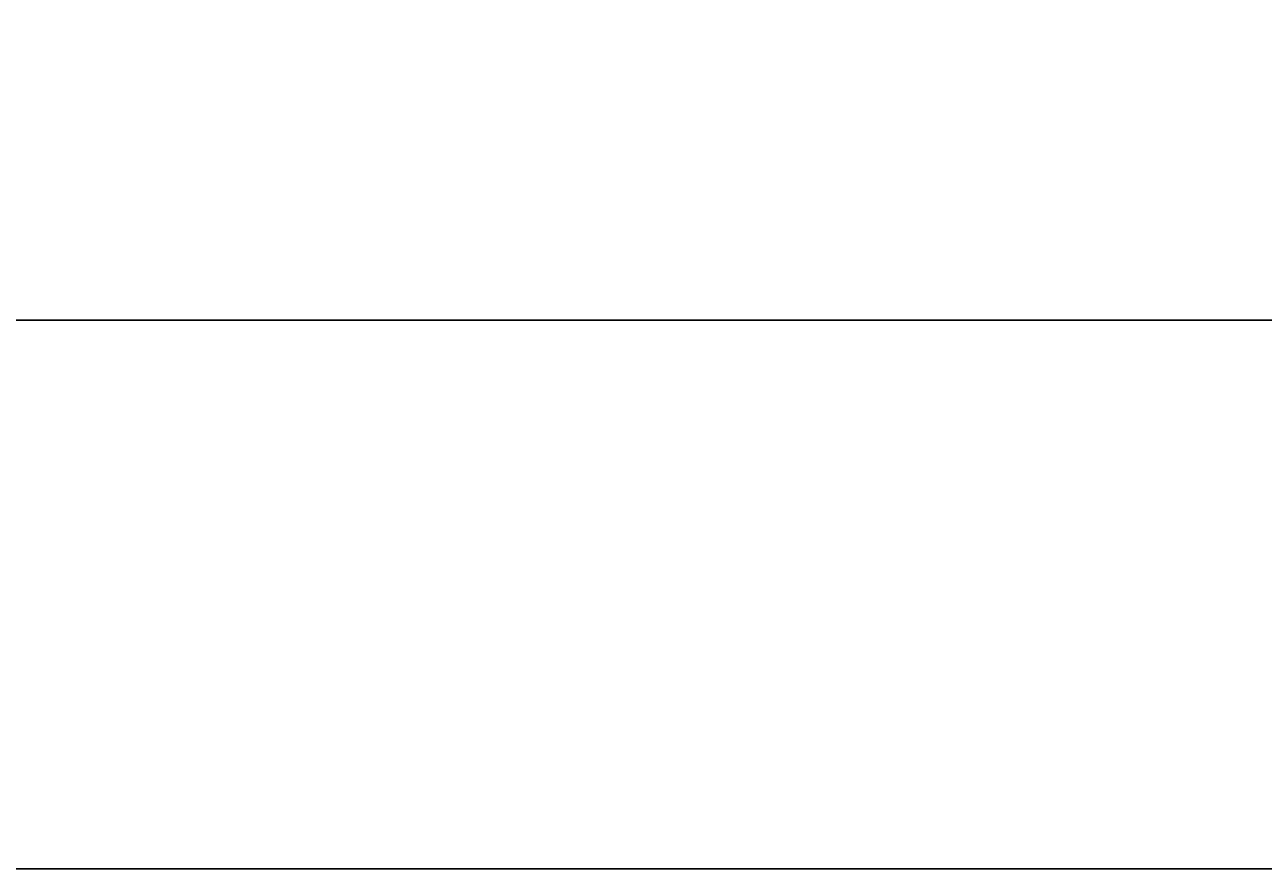
# Model space of a CAD drawing. Units: millimetres. Extents: x 27017497 to 27018854, y 7058029 to 7059154.
# Tile 63 of 91: x 27018319 to 27018462, y 7058029 to 7058126. Entities that reach past the tile are written whole.
import ezdxf

# ---------------------------------------------------------------- set-up
doc = ezdxf.new("R2010")
doc.units = ezdxf.units.MM
doc.layers.add('A-ANNO-DIMS', color=2, linetype='Continuous', lineweight=18)
doc.styles.get("Standard").update_dxf_attribs({"font": 'arial.ttf'})
doc.dimstyles.get("Standard").update_dxf_attribs({"dimtxt": 0.18, "dimasz": 0.18, "dimexe": 0.18, "dimexo": 0.0625, "dimgap": 0.09, "dimtad": 0, "dimtih": 1, "dimtoh": 1, "dimdec": 4, "dimzin": 0, "dimdsep": 46, "dimtxsty": 'Standard', "dimcen": 0.09, "dimadec": 0, "dimazin": 0, "dimtfac": 1, "dimtdec": 4, "dimtofl": 0, "dimtmove": 0, "dimatfit": 3, "dimfxl": 1, "dimtolj": 1, "dimtzin": 0, "dimarcsym": 0})

# ---------------------------------------------------------------- blocks, each defined once
blk = doc.blocks.new('*D47')
at = {"layer": 'A-ANNO-DIMS', "color": 0, "lineweight": -2, "transparency": 16777216}
for p, q in [((27017561.17, 7058294.35), (27017561.17, 7058028.6)), ((27018790.61, 7058294.35), (27018790.61, 7058028.6)), ((27017561.35, 7058028.78), (27018175.43, 7058028.78)), ((27018790.43, 7058028.78), (27018176.34, 7058028.78))]:
    blk.add_line(p, q, dxfattribs=at)
at = {"layer": 'A-ANNO-DIMS', "color": 0, "transparency": 16777216}
for points in [[(27017561.35, 7058028.81), (27017561.35, 7058028.75), (27017561.17, 7058028.78)], [(27018790.43, 7058028.81), (27018790.43, 7058028.75), (27018790.61, 7058028.78)]]:
    blk.add_solid(points, dxfattribs=at)
at = {"layer": 'Defpoints', "color": 0, "transparency": 16777216}
for p in [(27017561.17, 7058294.41), (27018790.61, 7058294.41), (27018790.61, 7058028.78)]:
    blk.add_point(p, dxfattribs=at)
at = {"layer": 'A-ANNO-DIMS', "color": 0, "transparency": 16777216, "insert": (27018175.89, 7058028.78), "char_height": 0.18, "attachment_point": 5}
blk.add_mtext('\\A1;1229.4', dxfattribs=at)
blk = doc.blocks.new('*D48')
at = {"layer": 'A-ANNO-DIMS', "color": 0, "lineweight": -2, "transparency": 16777216}
for p, q in [((27018463.5, 7058622.91), (27017497.54, 7058622.91)), ((27017497.72, 7058622.73), (27017497.72, 7058357.75)), ((27017497.72, 7058092.41), (27017497.72, 7058357.39)), ((27018555.13, 7058092.23), (27017497.54, 7058092.23))]:
    blk.add_line(p, q, dxfattribs=at)
at = {"layer": 'A-ANNO-DIMS', "color": 0, "transparency": 16777216}
for points in [[(27017497.69, 7058622.73), (27017497.75, 7058622.73), (27017497.72, 7058622.91)], [(27017497.69, 7058092.41), (27017497.75, 7058092.41), (27017497.72, 7058092.23)]]:
    blk.add_solid(points, dxfattribs=at)
at = {"layer": 'Defpoints', "color": 0, "transparency": 16777216}
for p in [(27018463.56, 7058622.91), (27017497.72, 7058092.23), (27018555.19, 7058092.23)]:
    blk.add_point(p, dxfattribs=at)
at = {"layer": 'A-ANNO-DIMS', "color": 0, "transparency": 16777216, "insert": (27017497.72, 7058357.57), "char_height": 0.18, "attachment_point": 5}
blk.add_mtext('\\A1;530.7', dxfattribs=at)

msp = doc.modelspace()

# ---------------------------------------------------------------- dimensions: what is measured, and where the dimension line sits
at = {"layer": 'A-ANNO-DIMS'}
dim = msp.add_linear_dim(base=(27017497.716, 7058092.23), p1=(27018463.561, 7058622.912), p2=(27018555.192, 7058092.23), angle=90, dimstyle='Standard', override={"dimdec": 1, "dimlfac": 1, "dimrnd": 0, "dimzin": 0, "dimdsep": 46, "dimlunit": 2}, dxfattribs=at)
dim.commit()
dim.dimension.update_dxf_attribs({"geometry": '*D48', "text_midpoint": (27017497.716, 7058357.571)})
dim = msp.add_linear_dim(base=(27018790.606, 7058028.78), p1=(27017561.166, 7058294.412), p2=(27018790.606, 7058294.412), dimstyle='Standard', override={"dimdec": 1, "dimlfac": 1, "dimrnd": 0, "dimzin": 0, "dimdsep": 46, "dimlunit": 2}, dxfattribs=at)
dim.commit()
dim.dimension.update_dxf_attribs({"geometry": '*D47', "text_midpoint": (27018175.886, 7058028.78)})

doc.saveas('drawing.dxf')
